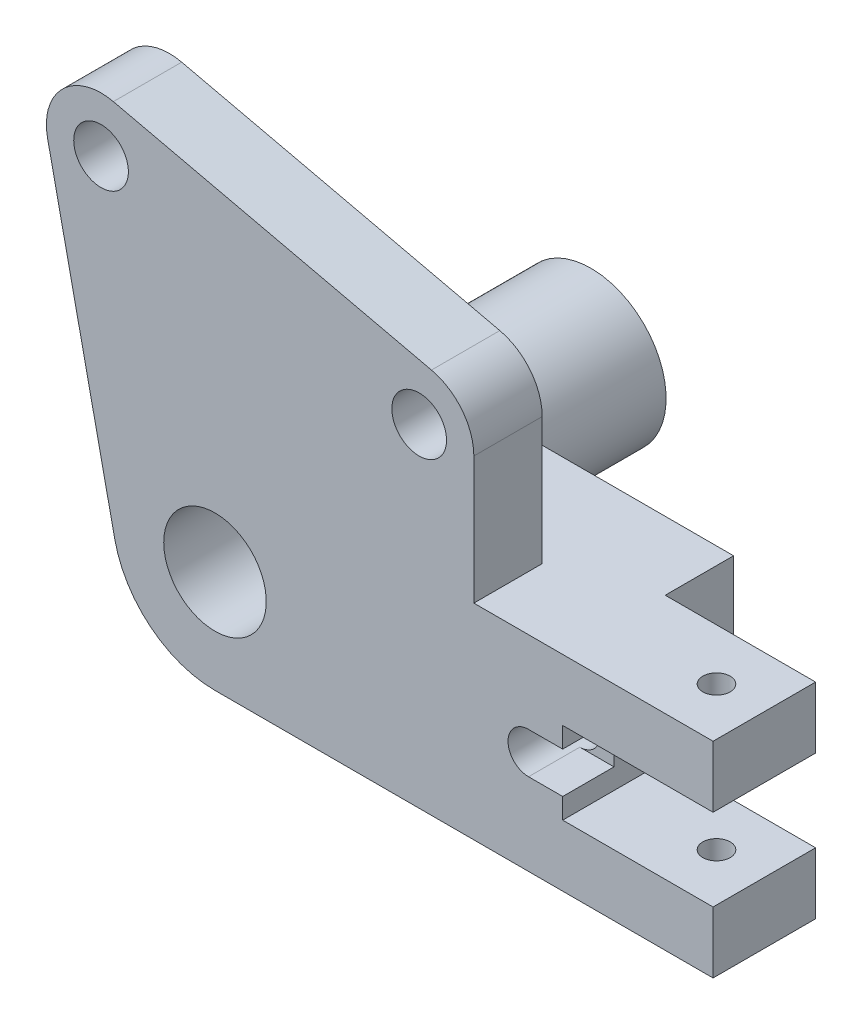
ISO-10303-21;
HEADER;
FILE_DESCRIPTION(('STEP AP214'),'2;1');
FILE_NAME('part.step','',(''),(''),'','','');
FILE_SCHEMA(('AUTOMOTIVE_DESIGN { 1 0 10303 214 1 1 1 1 }'));
ENDSEC;
DATA;
#1=APPLICATION_CONTEXT('core data for automotive mechanical design processes');
#2=APPLICATION_PROTOCOL_DEFINITION('international standard','automotive_design',2000,#1);
#3=PRODUCT_CONTEXT('',#1,'mechanical');
#4=PRODUCT('Part','Part','',(#3));
#5=PRODUCT_RELATED_PRODUCT_CATEGORY('part','',(#4));
#6=PRODUCT_DEFINITION_FORMATION('','',#4);
#7=PRODUCT_DEFINITION_CONTEXT('part definition',#1,'design');
#8=PRODUCT_DEFINITION('design','',#6,#7);
#9=PRODUCT_DEFINITION_SHAPE('','',#8);
#10=(LENGTH_UNIT() NAMED_UNIT(*) SI_UNIT(.MILLI.,.METRE.));
#11=(NAMED_UNIT(*) PLANE_ANGLE_UNIT() SI_UNIT($,.RADIAN.));
#12=(NAMED_UNIT(*) SI_UNIT($,.STERADIAN.) SOLID_ANGLE_UNIT());
#13=UNCERTAINTY_MEASURE_WITH_UNIT(LENGTH_MEASURE(1.E-05),#10,'distance_accuracy_value','');
#14=(GEOMETRIC_REPRESENTATION_CONTEXT(3) GLOBAL_UNCERTAINTY_ASSIGNED_CONTEXT((#13)) GLOBAL_UNIT_ASSIGNED_CONTEXT((#10,
#11,#12)) REPRESENTATION_CONTEXT('',''));
#15=CARTESIAN_POINT('',(0.,0.,0.));
#16=DIRECTION('',(0.,0.,1.));
#17=DIRECTION('',(1.,0.,0.));
#18=AXIS2_PLACEMENT_3D('',#15,#16,#17);
#19=CARTESIAN_POINT('',(-27.,15.,-5.));
#20=DIRECTION('',(0.,0.,1.));
#21=DIRECTION('',(1.,0.,0.));
#22=AXIS2_PLACEMENT_3D('',#19,#20,#21);
#23=CYLINDRICAL_SURFACE('',#22,3.);
#24=CARTESIAN_POINT('',(-27.,15.,10.));
#25=DIRECTION('',(0.,0.,1.));
#26=DIRECTION('',(1.,0.,0.));
#27=AXIS2_PLACEMENT_3D('',#24,#25,#26);
#28=CIRCLE('',#27,3.);
#29=CARTESIAN_POINT('',(-24.,15.,10.));
#30=VERTEX_POINT('',#29);
#31=EDGE_CURVE('E729',#30,#30,#28,.F.);
#32=ORIENTED_EDGE('',*,*,#31,.T.);
#33=EDGE_LOOP('',(#32));
#34=FACE_BOUND('',#33,.T.);
#35=DIRECTION('',(0.,0.,1.));
#36=VECTOR('',#35,1.);
#37=CARTESIAN_POINT('',(-27.,18.,17.5));
#38=LINE('',#37,#36);
#39=CARTESIAN_POINT('',(-27.,18.,17.5));
#40=VERTEX_POINT('',#39);
#41=CARTESIAN_POINT('',(-27.,18.,25.));
#42=VERTEX_POINT('',#41);
#43=EDGE_CURVE('E65',#40,#42,#38,.T.);
#44=ORIENTED_EDGE('',*,*,#43,.T.);
#45=CARTESIAN_POINT('',(-27.,15.,25.));
#46=DIRECTION('',(0.,0.,1.));
#47=DIRECTION('',(1.,0.,0.));
#48=AXIS2_PLACEMENT_3D('',#45,#46,#47);
#49=CIRCLE('',#48,3.);
#50=CARTESIAN_POINT('',(-27.,12.,25.));
#51=VERTEX_POINT('',#50);
#52=EDGE_CURVE('E377',#42,#51,#49,.T.);
#53=ORIENTED_EDGE('',*,*,#52,.T.);
#54=DIRECTION('',(0.,0.,1.));
#55=VECTOR('',#54,1.);
#56=CARTESIAN_POINT('',(-27.,12.,17.5));
#57=LINE('',#56,#55);
#58=CARTESIAN_POINT('',(-27.,12.,17.5));
#59=VERTEX_POINT('',#58);
#60=EDGE_CURVE('E739',#59,#51,#57,.T.);
#61=ORIENTED_EDGE('',*,*,#60,.F.);
#62=CARTESIAN_POINT('',(-27.,15.,17.5));
#63=DIRECTION('',(0.,0.,1.));
#64=DIRECTION('',(1.,0.,0.));
#65=AXIS2_PLACEMENT_3D('',#62,#63,#64);
#66=CIRCLE('',#65,3.);
#67=EDGE_CURVE('E274',#40,#59,#66,.F.);
#68=ORIENTED_EDGE('',*,*,#67,.F.);
#69=EDGE_LOOP('',(#44,#53,#61,#68));
#70=FACE_BOUND('',#69,.T.);
#71=ADVANCED_FACE('F39',(#34,#70),#23,.F.);
#72=CARTESIAN_POINT('',(-72.8737631464896,15.,0.));
#73=DIRECTION('',(0.,0.,-1.));
#74=DIRECTION('',(-1.,0.,0.));
#75=AXIS2_PLACEMENT_3D('',#72,#73,#74);
#76=PLANE('',#75);
#77=CARTESIAN_POINT('',(-27.,15.,0.));
#78=DIRECTION('',(0.,0.,-1.));
#79=DIRECTION('',(-1.,0.,0.));
#80=AXIS2_PLACEMENT_3D('',#77,#78,#79);
#81=CIRCLE('',#80,6.);
#82=CARTESIAN_POINT('',(-22.,11.6833752096446,0.));
#83=VERTEX_POINT('',#82);
#84=CARTESIAN_POINT('',(-22.,18.3166247903554,0.));
#85=VERTEX_POINT('',#84);
#86=EDGE_CURVE('E190',#83,#85,#81,.T.);
#87=ORIENTED_EDGE('',*,*,#86,.F.);
#88=DIRECTION('',(0.,1.,0.));
#89=VECTOR('',#88,1.);
#90=CARTESIAN_POINT('',(-22.,21.,0.));
#91=LINE('',#90,#89);
#92=CARTESIAN_POINT('',(-22.,0.,0.));
#93=VERTEX_POINT('',#92);
#94=EDGE_CURVE('E207',#93,#83,#91,.T.);
#95=ORIENTED_EDGE('',*,*,#94,.F.);
#96=DIRECTION('',(1.,0.,0.));
#97=VECTOR('',#96,1.);
#98=CARTESIAN_POINT('',(0.,0.,0.));
#99=LINE('',#98,#97);
#100=CARTESIAN_POINT('',(-72.8737631464896,0.,0.));
#101=VERTEX_POINT('',#100);
#102=EDGE_CURVE('E222',#101,#93,#99,.T.);
#103=ORIENTED_EDGE('',*,*,#102,.F.);
#104=CARTESIAN_POINT('',(-72.8737631464896,15.,0.));
#105=DIRECTION('',(0.,0.,1.));
#106=DIRECTION('',(-1.,0.,0.));
#107=AXIS2_PLACEMENT_3D('',#104,#105,#106);
#108=CIRCLE('',#107,15.);
#109=CARTESIAN_POINT('',(-87.5407993576508,11.857063669037,0.));
#110=VERTEX_POINT('',#109);
#111=EDGE_CURVE('E218',#110,#101,#108,.T.);
#112=ORIENTED_EDGE('',*,*,#111,.F.);
#113=DIRECTION('',(0.209529088730874,-0.977802414077409,0.));
#114=VECTOR('',#113,1.);
#115=CARTESIAN_POINT('',(-87.5407993576508,11.857063669037,0.));
#116=LINE('',#115,#114);
#117=CARTESIAN_POINT('',(-91.4285714285714,30.,0.));
#118=VERTEX_POINT('',#117);
#119=EDGE_CURVE('E217',#118,#110,#116,.T.);
#120=ORIENTED_EDGE('',*,*,#119,.F.);
#121=DIRECTION('',(-1.,0.,0.));
#122=VECTOR('',#121,1.);
#123=CARTESIAN_POINT('',(-35.,30.,0.));
#124=LINE('',#123,#122);
#125=CARTESIAN_POINT('',(-22.,30.,0.));
#126=VERTEX_POINT('',#125);
#127=EDGE_CURVE('E203',#126,#118,#124,.T.);
#128=ORIENTED_EDGE('',*,*,#127,.F.);
#129=EDGE_CURVE('E198',#85,#126,#91,.T.);
#130=ORIENTED_EDGE('',*,*,#129,.F.);
#131=EDGE_LOOP('',(#87,#95,#103,#112,#120,#128,#130));
#132=FACE_BOUND('',#131,.T.);
#133=CARTESIAN_POINT('',(-72.8737631464896,15.,0.));
#134=DIRECTION('',(0.,0.,-1.));
#135=DIRECTION('',(-1.,0.,0.));
#136=AXIS2_PLACEMENT_3D('',#133,#134,#135);
#137=CIRCLE('',#136,11.);
#138=CARTESIAN_POINT('',(-83.8737631464896,15.,0.));
#139=VERTEX_POINT('',#138);
#140=EDGE_CURVE('E315',#139,#139,#137,.T.);
#141=ORIENTED_EDGE('',*,*,#140,.F.);
#142=EDGE_LOOP('',(#141));
#143=FACE_BOUND('',#142,.T.);
#144=ADVANCED_FACE('F205',(#132,#143),#76,.T.);
#145=CARTESIAN_POINT('',(-35.,48.6358990374607,25.));
#146=DIRECTION('',(-1.,0.,0.));
#147=DIRECTION('',(0.,0.,1.));
#148=AXIS2_PLACEMENT_3D('',#145,#146,#147);
#149=PLANE('',#148);
#150=DIRECTION('',(0.,-1.,0.));
#151=VECTOR('',#150,1.);
#152=CARTESIAN_POINT('',(-35.,67.3763347936371,15.));
#153=LINE('',#152,#151);
#154=CARTESIAN_POINT('',(-35.,48.6358990374607,15.));
#155=VERTEX_POINT('',#154);
#156=CARTESIAN_POINT('',(-35.,30.,15.));
#157=VERTEX_POINT('',#156);
#158=EDGE_CURVE('E266',#155,#157,#153,.T.);
#159=ORIENTED_EDGE('',*,*,#158,.F.);
#160=DIRECTION('',(0.,0.,-1.));
#161=VECTOR('',#160,1.);
#162=CARTESIAN_POINT('',(-35.,48.6358990374607,25.));
#163=LINE('',#162,#161);
#164=CARTESIAN_POINT('',(-35.,48.6358990374607,25.));
#165=VERTEX_POINT('',#164);
#166=EDGE_CURVE('E243',#165,#155,#163,.T.);
#167=ORIENTED_EDGE('',*,*,#166,.F.);
#168=DIRECTION('',(0.,1.,0.));
#169=VECTOR('',#168,1.);
#170=CARTESIAN_POINT('',(-35.,48.6358990374607,25.));
#171=LINE('',#170,#169);
#172=CARTESIAN_POINT('',(-35.,30.,25.));
#173=VERTEX_POINT('',#172);
#174=EDGE_CURVE('E342',#173,#165,#171,.T.);
#175=ORIENTED_EDGE('',*,*,#174,.F.);
#176=DIRECTION('',(0.,0.,-1.));
#177=VECTOR('',#176,1.);
#178=CARTESIAN_POINT('',(-35.,30.,25.));
#179=LINE('',#178,#177);
#180=EDGE_CURVE('E246',#173,#157,#179,.T.);
#181=ORIENTED_EDGE('',*,*,#180,.T.);
#182=EDGE_LOOP('',(#159,#167,#175,#181));
#183=FACE_BOUND('',#182,.T.);
#184=ADVANCED_FACE('F435',(#183),#149,.F.);
#185=CARTESIAN_POINT('',(-43.,48.6358990374607,25.));
#186=DIRECTION('',(0.,0.,-1.));
#187=DIRECTION('',(-1.,0.,0.));
#188=AXIS2_PLACEMENT_3D('',#185,#186,#187);
#189=CYLINDRICAL_SURFACE('',#188,8.);
#190=CARTESIAN_POINT('',(-43.,48.6358990374607,15.));
#191=DIRECTION('',(0.,0.,-1.));
#192=DIRECTION('',(-1.,0.,0.));
#193=AXIS2_PLACEMENT_3D('',#190,#191,#192);
#194=CIRCLE('',#193,8.);
#195=CARTESIAN_POINT('',(-41.20112394641,56.4310286030177,15.));
#196=VERTEX_POINT('',#195);
#197=EDGE_CURVE('E324',#196,#155,#194,.T.);
#198=ORIENTED_EDGE('',*,*,#197,.F.);
#199=DIRECTION('',(0.,0.,-1.));
#200=VECTOR('',#199,1.);
#201=CARTESIAN_POINT('',(-41.20112394641,56.4310286030177,25.));
#202=LINE('',#201,#200);
#203=CARTESIAN_POINT('',(-41.20112394641,56.4310286030177,25.));
#204=VERTEX_POINT('',#203);
#205=EDGE_CURVE('E239',#204,#196,#202,.T.);
#206=ORIENTED_EDGE('',*,*,#205,.F.);
#207=CARTESIAN_POINT('',(-43.,48.6358990374607,25.));
#208=DIRECTION('',(0.,0.,1.));
#209=DIRECTION('',(1.,0.,0.));
#210=AXIS2_PLACEMENT_3D('',#207,#208,#209);
#211=CIRCLE('',#210,8.);
#212=EDGE_CURVE('E344',#165,#204,#211,.T.);
#213=ORIENTED_EDGE('',*,*,#212,.F.);
#214=ORIENTED_EDGE('',*,*,#166,.T.);
#215=EDGE_LOOP('',(#198,#206,#213,#214));
#216=FACE_BOUND('',#215,.T.);
#217=ADVANCED_FACE('F437',(#216),#189,.T.);
#218=CARTESIAN_POINT('',(-87.7430122231742,67.171464359194,25.));
#219=DIRECTION('',(-0.224859506698758,-0.97439119569462,0.));
#220=DIRECTION('',(0.97439119569462,-0.224859506698758,0.));
#221=AXIS2_PLACEMENT_3D('',#218,#219,#220);
#222=PLANE('',#221);
#223=DIRECTION('',(0.97439119569462,-0.224859506698758,0.));
#224=VECTOR('',#223,1.);
#225=CARTESIAN_POINT('',(-87.7430122231742,67.171464359194,15.));
#226=LINE('',#225,#224);
#227=CARTESIAN_POINT('',(-87.7430122231742,67.171464359194,15.));
#228=VERTEX_POINT('',#227);
#229=EDGE_CURVE('E322',#228,#196,#226,.T.);
#230=ORIENTED_EDGE('',*,*,#229,.F.);
#231=DIRECTION('',(0.,0.,-1.));
#232=VECTOR('',#231,1.);
#233=CARTESIAN_POINT('',(-87.7430122231742,67.171464359194,25.));
#234=LINE('',#233,#232);
#235=CARTESIAN_POINT('',(-87.7430122231742,67.171464359194,25.));
#236=VERTEX_POINT('',#235);
#237=EDGE_CURVE('E240',#236,#228,#234,.T.);
#238=ORIENTED_EDGE('',*,*,#237,.F.);
#239=DIRECTION('',(-0.97439119569462,0.224859506698758,0.));
#240=VECTOR('',#239,1.);
#241=CARTESIAN_POINT('',(-87.7430122231742,67.171464359194,25.));
#242=LINE('',#241,#240);
#243=EDGE_CURVE('E343',#204,#236,#242,.T.);
#244=ORIENTED_EDGE('',*,*,#243,.F.);
#245=ORIENTED_EDGE('',*,*,#205,.T.);
#246=EDGE_LOOP('',(#230,#238,#244,#245));
#247=FACE_BOUND('',#246,.T.);
#248=ADVANCED_FACE('F459',(#247),#222,.F.);
#249=CARTESIAN_POINT('',(-89.5418882767643,59.3763347936371,25.));
#250=DIRECTION('',(0.,0.,-1.));
#251=DIRECTION('',(-1.,0.,0.));
#252=AXIS2_PLACEMENT_3D('',#249,#250,#251);
#253=CYLINDRICAL_SURFACE('',#252,8.);
#254=CARTESIAN_POINT('',(-89.5418882767643,59.3763347936371,15.));
#255=DIRECTION('',(0.,0.,-1.));
#256=DIRECTION('',(-1.,0.,0.));
#257=AXIS2_PLACEMENT_3D('',#254,#255,#256);
#258=CIRCLE('',#257,8.);
#259=CARTESIAN_POINT('',(-97.3643075893836,57.70010208379,15.));
#260=VERTEX_POINT('',#259);
#261=EDGE_CURVE('E316',#260,#228,#258,.T.);
#262=ORIENTED_EDGE('',*,*,#261,.F.);
#263=DIRECTION('',(0.,0.,-1.));
#264=VECTOR('',#263,1.);
#265=CARTESIAN_POINT('',(-97.3643075893836,57.70010208379,25.));
#266=LINE('',#265,#264);
#267=CARTESIAN_POINT('',(-97.3643075893836,57.70010208379,25.));
#268=VERTEX_POINT('',#267);
#269=EDGE_CURVE('E234',#268,#260,#266,.T.);
#270=ORIENTED_EDGE('',*,*,#269,.F.);
#271=CARTESIAN_POINT('',(-89.5418882767643,59.3763347936371,25.));
#272=DIRECTION('',(0.,0.,1.));
#273=DIRECTION('',(1.,0.,0.));
#274=AXIS2_PLACEMENT_3D('',#271,#272,#273);
#275=CIRCLE('',#274,8.);
#276=EDGE_CURVE('E347',#236,#268,#275,.T.);
#277=ORIENTED_EDGE('',*,*,#276,.F.);
#278=ORIENTED_EDGE('',*,*,#237,.T.);
#279=EDGE_LOOP('',(#262,#270,#277,#278));
#280=FACE_BOUND('',#279,.T.);
#281=ADVANCED_FACE('F453',(#280),#253,.T.);
#282=CARTESIAN_POINT('',(-87.5407993576508,11.857063669037,25.));
#283=DIRECTION('',(0.977802414077409,0.209529088730874,0.));
#284=DIRECTION('',(-0.209529088730874,0.977802414077409,0.));
#285=AXIS2_PLACEMENT_3D('',#282,#283,#284);
#286=PLANE('',#285);
#287=DIRECTION('',(-0.209529088730874,0.977802414077409,0.));
#288=VECTOR('',#287,1.);
#289=CARTESIAN_POINT('',(-87.5407993576508,11.857063669037,15.));
#290=LINE('',#289,#288);
#291=CARTESIAN_POINT('',(-91.4285714285714,30.,15.));
#292=VERTEX_POINT('',#291);
#293=EDGE_CURVE('E296',#292,#260,#290,.T.);
#294=ORIENTED_EDGE('',*,*,#293,.F.);
#295=DIRECTION('',(0.,0.,1.));
#296=VECTOR('',#295,1.);
#297=CARTESIAN_POINT('',(-91.4285714285714,30.,25.));
#298=LINE('',#297,#296);
#299=EDGE_CURVE('E263',#118,#292,#298,.T.);
#300=ORIENTED_EDGE('',*,*,#299,.F.);
#301=ORIENTED_EDGE('',*,*,#119,.T.);
#302=DIRECTION('',(0.,0.,-1.));
#303=VECTOR('',#302,1.);
#304=CARTESIAN_POINT('',(-87.5407993576508,11.857063669037,25.));
#305=LINE('',#304,#303);
#306=CARTESIAN_POINT('',(-87.5407993576508,11.857063669037,25.));
#307=VERTEX_POINT('',#306);
#308=EDGE_CURVE('E233',#307,#110,#305,.T.);
#309=ORIENTED_EDGE('',*,*,#308,.F.);
#310=DIRECTION('',(0.209529088730874,-0.977802414077409,0.));
#311=VECTOR('',#310,1.);
#312=CARTESIAN_POINT('',(-87.5407993576508,11.857063669037,25.));
#313=LINE('',#312,#311);
#314=EDGE_CURVE('E294',#268,#307,#313,.T.);
#315=ORIENTED_EDGE('',*,*,#314,.F.);
#316=ORIENTED_EDGE('',*,*,#269,.T.);
#317=EDGE_LOOP('',(#294,#300,#301,#309,#315,#316));
#318=FACE_BOUND('',#317,.T.);
#319=ADVANCED_FACE('F295',(#318),#286,.F.);
#320=CARTESIAN_POINT('',(-89.5418882767643,59.3763347936371,25.));
#321=DIRECTION('',(0.,0.,-1.));
#322=DIRECTION('',(-1.,0.,0.));
#323=AXIS2_PLACEMENT_3D('',#320,#321,#322);
#324=CYLINDRICAL_SURFACE('',#323,4.00000000000001);
#325=CARTESIAN_POINT('',(-89.5418882767643,59.3763347936371,25.));
#326=DIRECTION('',(0.,0.,1.));
#327=DIRECTION('',(1.,0.,0.));
#328=AXIS2_PLACEMENT_3D('',#325,#326,#327);
#329=CIRCLE('',#328,4.00000000000001);
#330=CARTESIAN_POINT('',(-85.5418882767643,59.3763347936371,25.));
#331=VERTEX_POINT('',#330);
#332=EDGE_CURVE('E210',#331,#331,#329,.T.);
#333=ORIENTED_EDGE('',*,*,#332,.T.);
#334=EDGE_LOOP('',(#333));
#335=FACE_BOUND('',#334,.T.);
#336=CARTESIAN_POINT('',(-89.5418882767643,59.3763347936371,15.));
#337=DIRECTION('',(0.,0.,-1.));
#338=DIRECTION('',(-1.,0.,0.));
#339=AXIS2_PLACEMENT_3D('',#336,#337,#338);
#340=CIRCLE('',#339,4.00000000000001);
#341=CARTESIAN_POINT('',(-93.5418882767643,59.3763347936371,15.));
#342=VERTEX_POINT('',#341);
#343=EDGE_CURVE('E269',#342,#342,#340,.T.);
#344=ORIENTED_EDGE('',*,*,#343,.T.);
#345=EDGE_LOOP('',(#344));
#346=FACE_BOUND('',#345,.T.);
#347=ADVANCED_FACE('F451',(#335,#346),#324,.F.);
#348=CARTESIAN_POINT('',(-43.,48.6358990374607,25.));
#349=DIRECTION('',(0.,0.,-1.));
#350=DIRECTION('',(-1.,0.,0.));
#351=AXIS2_PLACEMENT_3D('',#348,#349,#350);
#352=CYLINDRICAL_SURFACE('',#351,4.);
#353=CARTESIAN_POINT('',(-43.,48.6358990374607,25.));
#354=DIRECTION('',(0.,0.,1.));
#355=DIRECTION('',(1.,0.,0.));
#356=AXIS2_PLACEMENT_3D('',#353,#354,#355);
#357=CIRCLE('',#356,4.);
#358=CARTESIAN_POINT('',(-39.,48.6358990374607,25.));
#359=VERTEX_POINT('',#358);
#360=EDGE_CURVE('E208',#359,#359,#357,.T.);
#361=ORIENTED_EDGE('',*,*,#360,.T.);
#362=EDGE_LOOP('',(#361));
#363=FACE_BOUND('',#362,.T.);
#364=CARTESIAN_POINT('',(-43.,48.6358990374607,15.));
#365=DIRECTION('',(0.,0.,-1.));
#366=DIRECTION('',(-1.,0.,0.));
#367=AXIS2_PLACEMENT_3D('',#364,#365,#366);
#368=CIRCLE('',#367,4.);
#369=CARTESIAN_POINT('',(-47.,48.6358990374607,15.));
#370=VERTEX_POINT('',#369);
#371=EDGE_CURVE('E265',#370,#370,#368,.T.);
#372=ORIENTED_EDGE('',*,*,#371,.T.);
#373=EDGE_LOOP('',(#372));
#374=FACE_BOUND('',#373,.T.);
#375=ADVANCED_FACE('F509',(#363,#374),#352,.F.);
#376=CARTESIAN_POINT('',(-72.8737631464896,15.,25.));
#377=DIRECTION('',(0.,0.,-1.));
#378=DIRECTION('',(-1.,0.,0.));
#379=AXIS2_PLACEMENT_3D('',#376,#377,#378);
#380=PLANE('',#379);
#381=CARTESIAN_POINT('',(-72.8737631464896,15.,25.));
#382=DIRECTION('',(0.,0.,-1.));
#383=DIRECTION('',(-1.,0.,0.));
#384=AXIS2_PLACEMENT_3D('',#381,#382,#383);
#385=CIRCLE('',#384,7.50000000000001);
#386=CARTESIAN_POINT('',(-80.3737631464896,15.,25.));
#387=VERTEX_POINT('',#386);
#388=EDGE_CURVE('E411',#387,#387,#385,.T.);
#389=ORIENTED_EDGE('',*,*,#388,.T.);
#390=EDGE_LOOP('',(#389));
#391=FACE_BOUND('',#390,.T.);
#392=ORIENTED_EDGE('',*,*,#52,.F.);
#393=DIRECTION('',(-1.,0.,0.));
#394=VECTOR('',#393,1.);
#395=CARTESIAN_POINT('',(-27.,18.,25.));
#396=LINE('',#395,#394);
#397=CARTESIAN_POINT('',(-22.,18.,25.));
#398=VERTEX_POINT('',#397);
#399=EDGE_CURVE('E732',#398,#42,#396,.T.);
#400=ORIENTED_EDGE('',*,*,#399,.F.);
#401=DIRECTION('',(0.,1.,0.));
#402=VECTOR('',#401,1.);
#403=CARTESIAN_POINT('',(-22.,21.,25.));
#404=LINE('',#403,#402);
#405=CARTESIAN_POINT('',(-22.,21.,25.));
#406=VERTEX_POINT('',#405);
#407=EDGE_CURVE('E332',#398,#406,#404,.T.);
#408=ORIENTED_EDGE('',*,*,#407,.T.);
#409=DIRECTION('',(1.,0.,0.));
#410=VECTOR('',#409,1.);
#411=CARTESIAN_POINT('',(0.,21.,25.));
#412=LINE('',#411,#410);
#413=CARTESIAN_POINT('',(0.,21.,25.));
#414=VERTEX_POINT('',#413);
#415=EDGE_CURVE('E333',#406,#414,#412,.T.);
#416=ORIENTED_EDGE('',*,*,#415,.T.);
#417=DIRECTION('',(0.,1.,0.));
#418=VECTOR('',#417,1.);
#419=CARTESIAN_POINT('',(0.,30.,25.));
#420=LINE('',#419,#418);
#421=CARTESIAN_POINT('',(0.,30.,25.));
#422=VERTEX_POINT('',#421);
#423=EDGE_CURVE('E340',#414,#422,#420,.T.);
#424=ORIENTED_EDGE('',*,*,#423,.T.);
#425=DIRECTION('',(-1.,0.,0.));
#426=VECTOR('',#425,1.);
#427=CARTESIAN_POINT('',(-35.,30.,25.));
#428=LINE('',#427,#426);
#429=EDGE_CURVE('E339',#422,#173,#428,.T.);
#430=ORIENTED_EDGE('',*,*,#429,.T.);
#431=ORIENTED_EDGE('',*,*,#174,.T.);
#432=ORIENTED_EDGE('',*,*,#212,.T.);
#433=ORIENTED_EDGE('',*,*,#243,.T.);
#434=ORIENTED_EDGE('',*,*,#276,.T.);
#435=ORIENTED_EDGE('',*,*,#314,.T.);
#436=CARTESIAN_POINT('',(-72.8737631464896,15.,25.));
#437=DIRECTION('',(0.,0.,1.));
#438=DIRECTION('',(-1.,0.,0.));
#439=AXIS2_PLACEMENT_3D('',#436,#437,#438);
#440=CIRCLE('',#439,15.);
#441=CARTESIAN_POINT('',(-72.8737631464896,0.,25.));
#442=VERTEX_POINT('',#441);
#443=EDGE_CURVE('E286',#307,#442,#440,.T.);
#444=ORIENTED_EDGE('',*,*,#443,.T.);
#445=DIRECTION('',(1.,0.,0.));
#446=VECTOR('',#445,1.);
#447=CARTESIAN_POINT('',(0.,0.,25.));
#448=LINE('',#447,#446);
#449=CARTESIAN_POINT('',(0.,0.,25.));
#450=VERTEX_POINT('',#449);
#451=EDGE_CURVE('E211',#442,#450,#448,.T.);
#452=ORIENTED_EDGE('',*,*,#451,.T.);
#453=DIRECTION('',(0.,1.,0.));
#454=VECTOR('',#453,1.);
#455=CARTESIAN_POINT('',(0.,9.,25.));
#456=LINE('',#455,#454);
#457=CARTESIAN_POINT('',(0.,9.,25.));
#458=VERTEX_POINT('',#457);
#459=EDGE_CURVE('E221',#450,#458,#456,.T.);
#460=ORIENTED_EDGE('',*,*,#459,.T.);
#461=DIRECTION('',(-1.,0.,0.));
#462=VECTOR('',#461,1.);
#463=CARTESIAN_POINT('',(-22.,9.,25.));
#464=LINE('',#463,#462);
#465=CARTESIAN_POINT('',(-22.,9.,25.));
#466=VERTEX_POINT('',#465);
#467=EDGE_CURVE('E328',#458,#466,#464,.T.);
#468=ORIENTED_EDGE('',*,*,#467,.T.);
#469=CARTESIAN_POINT('',(-22.,12.,25.));
#470=VERTEX_POINT('',#469);
#471=EDGE_CURVE('E335',#466,#470,#404,.T.);
#472=ORIENTED_EDGE('',*,*,#471,.T.);
#473=DIRECTION('',(1.,0.,0.));
#474=VECTOR('',#473,1.);
#475=CARTESIAN_POINT('',(-27.,12.,25.));
#476=LINE('',#475,#474);
#477=EDGE_CURVE('E366',#51,#470,#476,.T.);
#478=ORIENTED_EDGE('',*,*,#477,.F.);
#479=EDGE_LOOP('',(#392,#400,#408,#416,#424,#430,#431,#432,#433,#434,#435,#444,#452,#460,#468,
#472,#478));
#480=FACE_BOUND('',#479,.T.);
#481=ORIENTED_EDGE('',*,*,#332,.F.);
#482=EDGE_LOOP('',(#481));
#483=FACE_BOUND('',#482,.T.);
#484=ORIENTED_EDGE('',*,*,#360,.F.);
#485=EDGE_LOOP('',(#484));
#486=FACE_BOUND('',#485,.T.);
#487=ADVANCED_FACE('F352',(#391,#480,#483,#486),#380,.F.);
#488=CARTESIAN_POINT('',(0.,9.,25.));
#489=DIRECTION('',(-1.,0.,0.));
#490=DIRECTION('',(0.,0.,1.));
#491=AXIS2_PLACEMENT_3D('',#488,#489,#490);
#492=PLANE('',#491);
#493=DIRECTION('',(0.,0.,-1.));
#494=VECTOR('',#493,1.);
#495=CARTESIAN_POINT('',(0.,0.,25.));
#496=LINE('',#495,#494);
#497=CARTESIAN_POINT('',(0.,0.,10.));
#498=VERTEX_POINT('',#497);
#499=EDGE_CURVE('E223',#450,#498,#496,.T.);
#500=ORIENTED_EDGE('',*,*,#499,.T.);
#501=DIRECTION('',(0.,1.,0.));
#502=VECTOR('',#501,1.);
#503=CARTESIAN_POINT('',(0.,0.,10.));
#504=LINE('',#503,#502);
#505=CARTESIAN_POINT('',(0.,8.99999999999999,10.));
#506=VERTEX_POINT('',#505);
#507=EDGE_CURVE('E356',#498,#506,#504,.T.);
#508=ORIENTED_EDGE('',*,*,#507,.T.);
#509=DIRECTION('',(0.,0.,-1.));
#510=VECTOR('',#509,1.);
#511=CARTESIAN_POINT('',(0.,9.,25.));
#512=LINE('',#511,#510);
#513=EDGE_CURVE('E261',#458,#506,#512,.T.);
#514=ORIENTED_EDGE('',*,*,#513,.F.);
#515=ORIENTED_EDGE('',*,*,#459,.F.);
#516=EDGE_LOOP('',(#500,#508,#514,#515));
#517=FACE_BOUND('',#516,.T.);
#518=ADVANCED_FACE('F41',(#517),#492,.F.);
#519=CARTESIAN_POINT('',(-22.,9.,25.));
#520=DIRECTION('',(0.,-1.,0.));
#521=DIRECTION('',(1.,0.,0.));
#522=AXIS2_PLACEMENT_3D('',#519,#520,#521);
#523=PLANE('',#522);
#524=CARTESIAN_POINT('',(-7.,9.,17.5));
#525=DIRECTION('',(0.,-1.,0.));
#526=DIRECTION('',(1.,0.,0.));
#527=AXIS2_PLACEMENT_3D('',#524,#525,#526);
#528=CIRCLE('',#527,2.);
#529=CARTESIAN_POINT('',(-5.,9.,17.5));
#530=VERTEX_POINT('',#529);
#531=EDGE_CURVE('E394',#530,#530,#528,.T.);
#532=ORIENTED_EDGE('',*,*,#531,.T.);
#533=EDGE_LOOP('',(#532));
#534=FACE_BOUND('',#533,.T.);
#535=ORIENTED_EDGE('',*,*,#513,.T.);
#536=DIRECTION('',(-1.,0.,0.));
#537=VECTOR('',#536,1.);
#538=CARTESIAN_POINT('',(-22.,9.,10.));
#539=LINE('',#538,#537);
#540=CARTESIAN_POINT('',(-22.,9.,10.));
#541=VERTEX_POINT('',#540);
#542=EDGE_CURVE('E361',#506,#541,#539,.T.);
#543=ORIENTED_EDGE('',*,*,#542,.T.);
#544=DIRECTION('',(0.,0.,-1.));
#545=VECTOR('',#544,1.);
#546=CARTESIAN_POINT('',(-22.,9.,25.));
#547=LINE('',#546,#545);
#548=EDGE_CURVE('E259',#466,#541,#547,.T.);
#549=ORIENTED_EDGE('',*,*,#548,.F.);
#550=ORIENTED_EDGE('',*,*,#467,.F.);
#551=EDGE_LOOP('',(#535,#543,#549,#550));
#552=FACE_BOUND('',#551,.T.);
#553=ADVANCED_FACE('F363',(#534,#552),#523,.F.);
#554=CARTESIAN_POINT('',(-22.,21.,25.));
#555=DIRECTION('',(-1.,0.,0.));
#556=DIRECTION('',(0.,0.,1.));
#557=AXIS2_PLACEMENT_3D('',#554,#555,#556);
#558=PLANE('',#557);
#559=DIRECTION('',(0.,1.,0.));
#560=VECTOR('',#559,1.);
#561=CARTESIAN_POINT('',(-22.,21.,10.));
#562=LINE('',#561,#560);
#563=CARTESIAN_POINT('',(-22.,11.6833752096446,10.));
#564=VERTEX_POINT('',#563);
#565=CARTESIAN_POINT('',(-22.,18.3166247903554,10.));
#566=VERTEX_POINT('',#565);
#567=EDGE_CURVE('E50',#564,#566,#562,.T.);
#568=ORIENTED_EDGE('',*,*,#567,.T.);
#569=DIRECTION('',(0.,0.,-1.));
#570=VECTOR('',#569,1.);
#571=CARTESIAN_POINT('',(-22.,18.3166247903554,26.9705627484771));
#572=LINE('',#571,#570);
#573=EDGE_CURVE('E11',#566,#85,#572,.T.);
#574=ORIENTED_EDGE('',*,*,#573,.T.);
#575=ORIENTED_EDGE('',*,*,#129,.T.);
#576=DIRECTION('',(0.,0.,1.));
#577=VECTOR('',#576,1.);
#578=CARTESIAN_POINT('',(-22.,30.,10.));
#579=LINE('',#578,#577);
#580=CARTESIAN_POINT('',(-22.,30.,10.));
#581=VERTEX_POINT('',#580);
#582=EDGE_CURVE('E397',#126,#581,#579,.T.);
#583=ORIENTED_EDGE('',*,*,#582,.T.);
#584=DIRECTION('',(0.,1.,0.));
#585=VECTOR('',#584,1.);
#586=CARTESIAN_POINT('',(-22.,0.,10.));
#587=LINE('',#586,#585);
#588=CARTESIAN_POINT('',(-22.,21.,10.));
#589=VERTEX_POINT('',#588);
#590=EDGE_CURVE('E399',#589,#581,#587,.T.);
#591=ORIENTED_EDGE('',*,*,#590,.F.);
#592=DIRECTION('',(0.,0.,-1.));
#593=VECTOR('',#592,1.);
#594=CARTESIAN_POINT('',(-22.,21.,25.));
#595=LINE('',#594,#593);
#596=EDGE_CURVE('E253',#406,#589,#595,.T.);
#597=ORIENTED_EDGE('',*,*,#596,.F.);
#598=ORIENTED_EDGE('',*,*,#407,.F.);
#599=DIRECTION('',(0.,0.,-1.));
#600=VECTOR('',#599,1.);
#601=CARTESIAN_POINT('',(-22.,18.,25.));
#602=LINE('',#601,#600);
#603=CARTESIAN_POINT('',(-22.,18.,17.5));
#604=VERTEX_POINT('',#603);
#605=EDGE_CURVE('E376',#398,#604,#602,.T.);
#606=ORIENTED_EDGE('',*,*,#605,.T.);
#607=DIRECTION('',(0.,1.,0.));
#608=VECTOR('',#607,1.);
#609=CARTESIAN_POINT('',(-22.,21.,17.5));
#610=LINE('',#609,#608);
#611=CARTESIAN_POINT('',(-22.,12.,17.5));
#612=VERTEX_POINT('',#611);
#613=EDGE_CURVE('E375',#612,#604,#610,.T.);
#614=ORIENTED_EDGE('',*,*,#613,.F.);
#615=DIRECTION('',(0.,0.,1.));
#616=VECTOR('',#615,1.);
#617=CARTESIAN_POINT('',(-22.,12.,25.));
#618=LINE('',#617,#616);
#619=EDGE_CURVE('E369',#612,#470,#618,.T.);
#620=ORIENTED_EDGE('',*,*,#619,.T.);
#621=ORIENTED_EDGE('',*,*,#471,.F.);
#622=ORIENTED_EDGE('',*,*,#548,.T.);
#623=CARTESIAN_POINT('',(-22.,0.,10.));
#624=VERTEX_POINT('',#623);
#625=EDGE_CURVE('E403',#624,#541,#587,.T.);
#626=ORIENTED_EDGE('',*,*,#625,.F.);
#627=DIRECTION('',(0.,0.,1.));
#628=VECTOR('',#627,1.);
#629=CARTESIAN_POINT('',(-22.,0.,25.));
#630=LINE('',#629,#628);
#631=EDGE_CURVE('E272',#93,#624,#630,.T.);
#632=ORIENTED_EDGE('',*,*,#631,.F.);
#633=ORIENTED_EDGE('',*,*,#94,.T.);
#634=DIRECTION('',(0.,0.,-1.));
#635=VECTOR('',#634,1.);
#636=CARTESIAN_POINT('',(-22.,11.6833752096446,26.9705627484771));
#637=LINE('',#636,#635);
#638=EDGE_CURVE('E188',#83,#564,#637,.F.);
#639=ORIENTED_EDGE('',*,*,#638,.T.);
#640=EDGE_LOOP('',(#568,#574,#575,#583,#591,#597,#598,#606,#614,#620,#621,#622,#626,#632,#633,#639));
#641=FACE_BOUND('',#640,.T.);
#642=ADVANCED_FACE('F197',(#641),#558,.F.);
#643=CARTESIAN_POINT('',(0.,21.,25.));
#644=DIRECTION('',(0.,1.,0.));
#645=DIRECTION('',(-1.,0.,0.));
#646=AXIS2_PLACEMENT_3D('',#643,#644,#645);
#647=PLANE('',#646);
#648=CARTESIAN_POINT('',(-7.,21.,17.5));
#649=DIRECTION('',(0.,1.,0.));
#650=DIRECTION('',(-1.,0.,0.));
#651=AXIS2_PLACEMENT_3D('',#648,#649,#650);
#652=CIRCLE('',#651,2.);
#653=CARTESIAN_POINT('',(-9.,21.,17.5));
#654=VERTEX_POINT('',#653);
#655=EDGE_CURVE('E389',#654,#654,#652,.T.);
#656=ORIENTED_EDGE('',*,*,#655,.T.);
#657=EDGE_LOOP('',(#656));
#658=FACE_BOUND('',#657,.T.);
#659=ORIENTED_EDGE('',*,*,#596,.T.);
#660=DIRECTION('',(1.,0.,0.));
#661=VECTOR('',#660,1.);
#662=CARTESIAN_POINT('',(0.,21.,10.));
#663=LINE('',#662,#661);
#664=CARTESIAN_POINT('',(0.,21.,10.));
#665=VERTEX_POINT('',#664);
#666=EDGE_CURVE('E401',#589,#665,#663,.T.);
#667=ORIENTED_EDGE('',*,*,#666,.T.);
#668=DIRECTION('',(0.,0.,-1.));
#669=VECTOR('',#668,1.);
#670=CARTESIAN_POINT('',(0.,21.,25.));
#671=LINE('',#670,#669);
#672=EDGE_CURVE('E255',#414,#665,#671,.T.);
#673=ORIENTED_EDGE('',*,*,#672,.F.);
#674=ORIENTED_EDGE('',*,*,#415,.F.);
#675=EDGE_LOOP('',(#659,#667,#673,#674));
#676=FACE_BOUND('',#675,.T.);
#677=ADVANCED_FACE('F475',(#658,#676),#647,.F.);
#678=CARTESIAN_POINT('',(0.,30.,25.));
#679=DIRECTION('',(-1.,0.,0.));
#680=DIRECTION('',(0.,0.,1.));
#681=AXIS2_PLACEMENT_3D('',#678,#679,#680);
#682=PLANE('',#681);
#683=ORIENTED_EDGE('',*,*,#672,.T.);
#684=CARTESIAN_POINT('',(0.,30.,10.));
#685=VERTEX_POINT('',#684);
#686=EDGE_CURVE('E404',#665,#685,#504,.T.);
#687=ORIENTED_EDGE('',*,*,#686,.T.);
#688=DIRECTION('',(0.,0.,-1.));
#689=VECTOR('',#688,1.);
#690=CARTESIAN_POINT('',(0.,30.,25.));
#691=LINE('',#690,#689);
#692=EDGE_CURVE('E248',#422,#685,#691,.T.);
#693=ORIENTED_EDGE('',*,*,#692,.F.);
#694=ORIENTED_EDGE('',*,*,#423,.F.);
#695=EDGE_LOOP('',(#683,#687,#693,#694));
#696=FACE_BOUND('',#695,.T.);
#697=ADVANCED_FACE('F466',(#696),#682,.F.);
#698=CARTESIAN_POINT('',(-35.,30.,25.));
#699=DIRECTION('',(0.,-1.,0.));
#700=DIRECTION('',(1.,0.,0.));
#701=AXIS2_PLACEMENT_3D('',#698,#699,#700);
#702=PLANE('',#701);
#703=CARTESIAN_POINT('',(-7.,30.,17.5));
#704=DIRECTION('',(0.,1.,0.));
#705=DIRECTION('',(-1.,0.,0.));
#706=AXIS2_PLACEMENT_3D('',#703,#704,#705);
#707=CIRCLE('',#706,2.);
#708=CARTESIAN_POINT('',(-9.,30.,17.5));
#709=VERTEX_POINT('',#708);
#710=EDGE_CURVE('E381',#709,#709,#707,.T.);
#711=ORIENTED_EDGE('',*,*,#710,.F.);
#712=EDGE_LOOP('',(#711));
#713=FACE_BOUND('',#712,.T.);
#714=ORIENTED_EDGE('',*,*,#692,.T.);
#715=DIRECTION('',(1.,0.,0.));
#716=VECTOR('',#715,1.);
#717=CARTESIAN_POINT('',(0.,30.,10.));
#718=LINE('',#717,#716);
#719=EDGE_CURVE('E396',#581,#685,#718,.T.);
#720=ORIENTED_EDGE('',*,*,#719,.F.);
#721=ORIENTED_EDGE('',*,*,#582,.F.);
#722=ORIENTED_EDGE('',*,*,#127,.T.);
#723=ORIENTED_EDGE('',*,*,#299,.T.);
#724=DIRECTION('',(1.,0.,0.));
#725=VECTOR('',#724,1.);
#726=CARTESIAN_POINT('',(-35.,30.,15.));
#727=LINE('',#726,#725);
#728=EDGE_CURVE('E302',#292,#157,#727,.T.);
#729=ORIENTED_EDGE('',*,*,#728,.T.);
#730=ORIENTED_EDGE('',*,*,#180,.F.);
#731=ORIENTED_EDGE('',*,*,#429,.F.);
#732=EDGE_LOOP('',(#714,#720,#721,#722,#723,#729,#730,#731));
#733=FACE_BOUND('',#732,.T.);
#734=ADVANCED_FACE('F305',(#713,#733),#702,.F.);
#735=CARTESIAN_POINT('',(-72.8737631464896,15.,25.));
#736=DIRECTION('',(0.,0.,-1.));
#737=DIRECTION('',(-1.,0.,0.));
#738=AXIS2_PLACEMENT_3D('',#735,#736,#737);
#739=CYLINDRICAL_SURFACE('',#738,15.);
#740=ORIENTED_EDGE('',*,*,#111,.T.);
#741=DIRECTION('',(0.,0.,-1.));
#742=VECTOR('',#741,1.);
#743=CARTESIAN_POINT('',(-72.8737631464896,0.,25.));
#744=LINE('',#743,#742);
#745=EDGE_CURVE('E226',#442,#101,#744,.T.);
#746=ORIENTED_EDGE('',*,*,#745,.F.);
#747=ORIENTED_EDGE('',*,*,#443,.F.);
#748=ORIENTED_EDGE('',*,*,#308,.T.);
#749=EDGE_LOOP('',(#740,#746,#747,#748));
#750=FACE_BOUND('',#749,.T.);
#751=ADVANCED_FACE('F289',(#750),#739,.T.);
#752=CARTESIAN_POINT('',(0.,0.,25.));
#753=DIRECTION('',(0.,1.,0.));
#754=DIRECTION('',(0.,0.,1.));
#755=AXIS2_PLACEMENT_3D('',#752,#753,#754);
#756=PLANE('',#755);
#757=CARTESIAN_POINT('',(-7.,0.,17.5));
#758=DIRECTION('',(0.,1.,0.));
#759=DIRECTION('',(-1.,0.,0.));
#760=AXIS2_PLACEMENT_3D('',#757,#758,#759);
#761=CIRCLE('',#760,2.);
#762=CARTESIAN_POINT('',(-9.,0.,17.5));
#763=VERTEX_POINT('',#762);
#764=EDGE_CURVE('E383',#763,#763,#761,.T.);
#765=ORIENTED_EDGE('',*,*,#764,.T.);
#766=EDGE_LOOP('',(#765));
#767=FACE_BOUND('',#766,.T.);
#768=ORIENTED_EDGE('',*,*,#631,.T.);
#769=DIRECTION('',(1.,0.,0.));
#770=VECTOR('',#769,1.);
#771=CARTESIAN_POINT('',(0.,0.,10.));
#772=LINE('',#771,#770);
#773=EDGE_CURVE('E353',#624,#498,#772,.T.);
#774=ORIENTED_EDGE('',*,*,#773,.T.);
#775=ORIENTED_EDGE('',*,*,#499,.F.);
#776=ORIENTED_EDGE('',*,*,#451,.F.);
#777=ORIENTED_EDGE('',*,*,#745,.T.);
#778=ORIENTED_EDGE('',*,*,#102,.T.);
#779=EDGE_LOOP('',(#768,#774,#775,#776,#777,#778));
#780=FACE_BOUND('',#779,.T.);
#781=ADVANCED_FACE('F281',(#767,#780),#756,.F.);
#782=CARTESIAN_POINT('',(-35.,67.3763347936371,15.));
#783=DIRECTION('',(0.,0.,-1.));
#784=DIRECTION('',(-1.,0.,0.));
#785=AXIS2_PLACEMENT_3D('',#782,#783,#784);
#786=PLANE('',#785);
#787=ORIENTED_EDGE('',*,*,#343,.F.);
#788=EDGE_LOOP('',(#787));
#789=FACE_BOUND('',#788,.T.);
#790=ORIENTED_EDGE('',*,*,#371,.F.);
#791=EDGE_LOOP('',(#790));
#792=FACE_BOUND('',#791,.T.);
#793=ORIENTED_EDGE('',*,*,#197,.T.);
#794=ORIENTED_EDGE('',*,*,#158,.T.);
#795=ORIENTED_EDGE('',*,*,#728,.F.);
#796=ORIENTED_EDGE('',*,*,#293,.T.);
#797=ORIENTED_EDGE('',*,*,#261,.T.);
#798=ORIENTED_EDGE('',*,*,#229,.T.);
#799=EDGE_LOOP('',(#793,#794,#795,#796,#797,#798));
#800=FACE_BOUND('',#799,.T.);
#801=ADVANCED_FACE('F306',(#789,#792,#800),#786,.T.);
#802=CARTESIAN_POINT('',(-72.8737631464896,15.,-30.));
#803=DIRECTION('',(0.,0.,1.));
#804=DIRECTION('',(1.,0.,0.));
#805=AXIS2_PLACEMENT_3D('',#802,#803,#804);
#806=CYLINDRICAL_SURFACE('',#805,11.);
#807=CARTESIAN_POINT('',(-72.8737631464896,15.,-30.));
#808=DIRECTION('',(0.,0.,-1.));
#809=DIRECTION('',(-1.,0.,0.));
#810=AXIS2_PLACEMENT_3D('',#807,#808,#809);
#811=CIRCLE('',#810,11.);
#812=CARTESIAN_POINT('',(-83.8737631464896,15.,-30.));
#813=VERTEX_POINT('',#812);
#814=EDGE_CURVE('E308',#813,#813,#811,.T.);
#815=ORIENTED_EDGE('',*,*,#814,.F.);
#816=EDGE_LOOP('',(#815));
#817=FACE_BOUND('',#816,.T.);
#818=ORIENTED_EDGE('',*,*,#140,.T.);
#819=EDGE_LOOP('',(#818));
#820=FACE_BOUND('',#819,.T.);
#821=ADVANCED_FACE('F422',(#817,#820),#806,.T.);
#822=CARTESIAN_POINT('',(-72.8737631464896,15.,-30.));
#823=DIRECTION('',(0.,0.,-1.));
#824=DIRECTION('',(-1.,0.,0.));
#825=AXIS2_PLACEMENT_3D('',#822,#823,#824);
#826=PLANE('',#825);
#827=CARTESIAN_POINT('',(-72.8737631464896,15.,-30.));
#828=DIRECTION('',(0.,0.,-1.));
#829=DIRECTION('',(-1.,0.,0.));
#830=AXIS2_PLACEMENT_3D('',#827,#828,#829);
#831=CIRCLE('',#830,7.50000000000001);
#832=CARTESIAN_POINT('',(-80.3737631464896,15.,-30.));
#833=VERTEX_POINT('',#832);
#834=EDGE_CURVE('E408',#833,#833,#831,.T.);
#835=ORIENTED_EDGE('',*,*,#834,.F.);
#836=EDGE_LOOP('',(#835));
#837=FACE_BOUND('',#836,.T.);
#838=ORIENTED_EDGE('',*,*,#814,.T.);
#839=EDGE_LOOP('',(#838));
#840=FACE_BOUND('',#839,.T.);
#841=ADVANCED_FACE('F416',(#837,#840),#826,.T.);
#842=CARTESIAN_POINT('',(-72.8737631464896,15.,25.));
#843=DIRECTION('',(0.,0.,-1.));
#844=DIRECTION('',(-1.,0.,0.));
#845=AXIS2_PLACEMENT_3D('',#842,#843,#844);
#846=CYLINDRICAL_SURFACE('',#845,7.50000000000001);
#847=ORIENTED_EDGE('',*,*,#388,.F.);
#848=EDGE_LOOP('',(#847));
#849=FACE_BOUND('',#848,.T.);
#850=ORIENTED_EDGE('',*,*,#834,.T.);
#851=EDGE_LOOP('',(#850));
#852=FACE_BOUND('',#851,.T.);
#853=ADVANCED_FACE('F420',(#849,#852),#846,.F.);
#854=CARTESIAN_POINT('',(0.,0.,10.));
#855=DIRECTION('',(0.,0.,1.));
#856=DIRECTION('',(1.,0.,0.));
#857=AXIS2_PLACEMENT_3D('',#854,#855,#856);
#858=PLANE('',#857);
#859=ORIENTED_EDGE('',*,*,#507,.F.);
#860=ORIENTED_EDGE('',*,*,#773,.F.);
#861=ORIENTED_EDGE('',*,*,#625,.T.);
#862=ORIENTED_EDGE('',*,*,#542,.F.);
#863=EDGE_LOOP('',(#859,#860,#861,#862));
#864=FACE_BOUND('',#863,.T.);
#865=ADVANCED_FACE('F496',(#864),#858,.F.);
#866=ORIENTED_EDGE('',*,*,#590,.T.);
#867=ORIENTED_EDGE('',*,*,#719,.T.);
#868=ORIENTED_EDGE('',*,*,#686,.F.);
#869=ORIENTED_EDGE('',*,*,#666,.F.);
#870=EDGE_LOOP('',(#866,#867,#868,#869));
#871=FACE_BOUND('',#870,.T.);
#872=ADVANCED_FACE('F486',(#871),#858,.F.);
#873=CARTESIAN_POINT('',(-7.,0.,17.5));
#874=DIRECTION('',(0.,1.,0.));
#875=DIRECTION('',(-1.,0.,0.));
#876=AXIS2_PLACEMENT_3D('',#873,#874,#875);
#877=CYLINDRICAL_SURFACE('',#876,2.);
#878=ORIENTED_EDGE('',*,*,#764,.F.);
#879=EDGE_LOOP('',(#878));
#880=FACE_BOUND('',#879,.T.);
#881=ORIENTED_EDGE('',*,*,#531,.F.);
#882=EDGE_LOOP('',(#881));
#883=FACE_BOUND('',#882,.T.);
#884=ADVANCED_FACE('F483',(#880,#883),#877,.F.);
#885=ORIENTED_EDGE('',*,*,#710,.T.);
#886=EDGE_LOOP('',(#885));
#887=FACE_BOUND('',#886,.T.);
#888=ORIENTED_EDGE('',*,*,#655,.F.);
#889=EDGE_LOOP('',(#888));
#890=FACE_BOUND('',#889,.T.);
#891=ADVANCED_FACE('F487',(#887,#890),#877,.F.);
#892=CARTESIAN_POINT('',(-27.,18.,17.5));
#893=DIRECTION('',(0.,1.,0.));
#894=DIRECTION('',(0.,0.,1.));
#895=AXIS2_PLACEMENT_3D('',#892,#893,#894);
#896=PLANE('',#895);
#897=ORIENTED_EDGE('',*,*,#399,.T.);
#898=ORIENTED_EDGE('',*,*,#43,.F.);
#899=DIRECTION('',(-1.,0.,0.));
#900=VECTOR('',#899,1.);
#901=CARTESIAN_POINT('',(-27.,18.,17.5));
#902=LINE('',#901,#900);
#903=EDGE_CURVE('E737',#604,#40,#902,.T.);
#904=ORIENTED_EDGE('',*,*,#903,.F.);
#905=ORIENTED_EDGE('',*,*,#605,.F.);
#906=EDGE_LOOP('',(#897,#898,#904,#905));
#907=FACE_BOUND('',#906,.T.);
#908=ADVANCED_FACE('F494',(#907),#896,.F.);
#909=CARTESIAN_POINT('',(-27.,12.,17.5));
#910=DIRECTION('',(0.,-1.,0.));
#911=DIRECTION('',(0.,0.,-1.));
#912=AXIS2_PLACEMENT_3D('',#909,#910,#911);
#913=PLANE('',#912);
#914=DIRECTION('',(1.,0.,0.));
#915=VECTOR('',#914,1.);
#916=CARTESIAN_POINT('',(-27.,12.,17.5));
#917=LINE('',#916,#915);
#918=EDGE_CURVE('E733',#59,#612,#917,.T.);
#919=ORIENTED_EDGE('',*,*,#918,.F.);
#920=ORIENTED_EDGE('',*,*,#60,.T.);
#921=ORIENTED_EDGE('',*,*,#477,.T.);
#922=ORIENTED_EDGE('',*,*,#619,.F.);
#923=EDGE_LOOP('',(#919,#920,#921,#922));
#924=FACE_BOUND('',#923,.T.);
#925=ADVANCED_FACE('F538',(#924),#913,.F.);
#926=CARTESIAN_POINT('',(0.,0.,17.5));
#927=DIRECTION('',(0.,0.,1.));
#928=DIRECTION('',(1.,0.,0.));
#929=AXIS2_PLACEMENT_3D('',#926,#927,#928);
#930=PLANE('',#929);
#931=ORIENTED_EDGE('',*,*,#613,.T.);
#932=ORIENTED_EDGE('',*,*,#903,.T.);
#933=ORIENTED_EDGE('',*,*,#67,.T.);
#934=ORIENTED_EDGE('',*,*,#918,.T.);
#935=EDGE_LOOP('',(#931,#932,#933,#934));
#936=FACE_BOUND('',#935,.T.);
#937=ADVANCED_FACE('F546',(#936),#930,.T.);
#938=CARTESIAN_POINT('',(0.,0.,10.));
#939=DIRECTION('',(0.,0.,1.));
#940=DIRECTION('',(1.,0.,0.));
#941=AXIS2_PLACEMENT_3D('',#938,#939,#940);
#942=PLANE('',#941);
#943=CARTESIAN_POINT('',(-27.,15.,10.));
#944=DIRECTION('',(0.,0.,1.));
#945=DIRECTION('',(1.,0.,0.));
#946=AXIS2_PLACEMENT_3D('',#943,#944,#945);
#947=CIRCLE('',#946,6.);
#948=EDGE_CURVE('E53',#564,#566,#947,.F.);
#949=ORIENTED_EDGE('',*,*,#948,.T.);
#950=ORIENTED_EDGE('',*,*,#567,.F.);
#951=EDGE_LOOP('',(#949,#950));
#952=FACE_BOUND('',#951,.T.);
#953=ORIENTED_EDGE('',*,*,#31,.F.);
#954=EDGE_LOOP('',(#953));
#955=FACE_BOUND('',#954,.T.);
#956=ADVANCED_FACE('F554',(#952,#955),#942,.F.);
#957=CARTESIAN_POINT('',(-27.,15.,26.9705627484771));
#958=DIRECTION('',(0.,0.,-1.));
#959=DIRECTION('',(-1.,0.,0.));
#960=AXIS2_PLACEMENT_3D('',#957,#958,#959);
#961=CYLINDRICAL_SURFACE('',#960,6.);
#962=ORIENTED_EDGE('',*,*,#948,.F.);
#963=ORIENTED_EDGE('',*,*,#638,.F.);
#964=ORIENTED_EDGE('',*,*,#86,.T.);
#965=ORIENTED_EDGE('',*,*,#573,.F.);
#966=EDGE_LOOP('',(#962,#963,#964,#965));
#967=FACE_BOUND('',#966,.T.);
#968=ADVANCED_FACE('F189',(#967),#961,.F.);
#969=CLOSED_SHELL('',(#71,#144,#184,#217,#248,#281,#319,#347,#375,#487,#518,#553,#642,#677,#697,
#734,#751,#781,#801,#821,#841,#853,#865,#872,#884,#891,#908,#925,#937,#956,#968));
#970=MANIFOLD_SOLID_BREP('B2',#969);
#971=ADVANCED_BREP_SHAPE_REPRESENTATION('',(#18,#970),#14);
#972=SHAPE_DEFINITION_REPRESENTATION(#9,#971);
ENDSEC;
END-ISO-10303-21;
